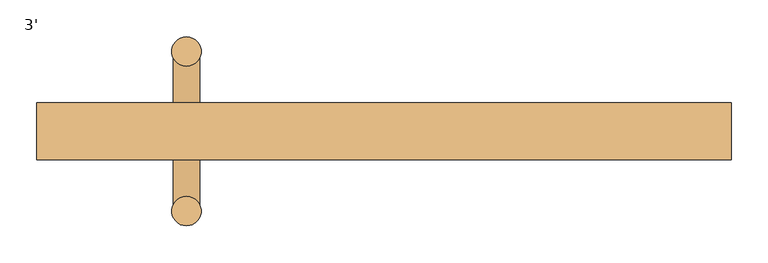
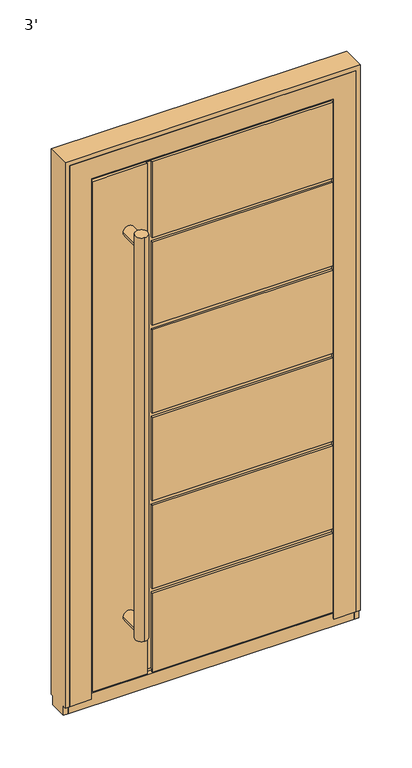
"""IFC4 building model written with IfcOpenShell, lengths in millimetres: door geometry, 3'."""

from ifc_helpers import new_model, si_unit, point, frame, frame_2d, origin, place, context, project, spatial, circle_curve, trimmed, segment, composite_curve, outline, extrude, faceted_brep, source, transform, mapped, element, save


def door_3_ad1505b7(model_context):
    return source(origin(), model_context, "Body", "SolidModel", [
        extrude(outline(composite_curve([segment(trimmed(circle_curve(frame_2d((-268.65, -90.8003001)), 20.0), [point((-268.65, -70.8003001))], [point((-268.65, -110.8003001))], False, "CARTESIAN"), True, "CONTINUOUS"), segment(trimmed(circle_curve(frame_2d((-268.65, -90.8003001)), 20.0), [point((-268.65, -110.8003001))], [point((-268.65, -70.8003001))], False, "CARTESIAN"), True, "CONTINUOUS")], self_intersect=False)), frame((0.0, 0.0, 210.0000003), z_axis=(0.0, 0.0, 1.0), x_axis=(1.0, 0.0, 0.0)), (0.0, 0.0, 1.0), 1363.8),
        extrude(outline(composite_curve([segment(trimmed(circle_curve(frame_2d((-268.65, 126.2003001)), 20.0), [point((-268.65, 146.2003001))], [point((-268.65, 106.2003001))], False, "CARTESIAN"), True, "CONTINUOUS"), segment(trimmed(circle_curve(frame_2d((-268.65, 126.2003001)), 20.0), [point((-268.65, 106.2003001))], [point((-268.65, 146.2003001))], False, "CARTESIAN"), True, "CONTINUOUS")], self_intersect=False)), frame((0.0, 0.0, 210.0000003), z_axis=(0.0, 0.0, 1.0), x_axis=(1.0, 0.0, 0.0)), (0.0, 0.0, 1.0), 1363.8),
        extrude(outline(composite_curve([segment(trimmed(circle_curve(frame_2d((241.9000003, -268.65)), 18.0), [point((241.9000003, -286.65))], [point((241.9000003, -250.65))], False, "CARTESIAN"), True, "CONTINUOUS"), segment(trimmed(circle_curve(frame_2d((241.9000003, -268.65)), 18.0), [point((241.9000003, -250.65))], [point((241.9000003, -286.65))], False, "CARTESIAN"), True, "CONTINUOUS")], self_intersect=False)), frame((0.0, -90.8, 0.0), z_axis=(0.0, 1.0, 0.0), x_axis=(0.0, 0.0, 1.0)), (0.0, 0.0, 1.0), 217.0),
        extrude(outline(composite_curve([segment(trimmed(circle_curve(frame_2d((1541.9000003, -268.65)), 18.0), [point((1541.9000003, -286.65))], [point((1541.9000003, -250.65))], False, "CARTESIAN"), True, "CONTINUOUS"), segment(trimmed(circle_curve(frame_2d((1541.9000003, -268.65)), 18.0), [point((1541.9000003, -250.65))], [point((1541.9000003, -286.65))], False, "CARTESIAN"), True, "CONTINUOUS")], self_intersect=False)), frame((0.0, -90.8, 0.0), z_axis=(0.0, 1.0, 0.0), x_axis=(0.0, 0.0, 1.0)), (0.0, 0.0, 1.0), 217.0),
        faceted_brep([(-193.65, -13.8, 306.466667), (-193.65, -13.8, 587.9333337), (383.65, -13.8, 587.9333337), (383.65, -13.8, 602.9333337), (-193.65, -13.8, 602.9333337), (-193.65, -13.8, 884.4000004), (383.65, -13.8, 884.4000004), (383.65, -13.8, 899.4000004), (-193.65, -13.8, 899.4000004), (-193.65, -13.8, 1180.866667), (383.65, -13.8, 1180.866667), (383.65, -13.8, 1195.866667), (-193.65, -13.8, 1195.866667), (-193.65, -13.8, 1477.3333337), (383.65, -13.8, 1477.3333337), (383.65, -13.8, 1492.3333337), (-193.65, -13.8, 1492.3333337), (-193.65, -13.8, 1748.8000003), (-208.65, -13.8, 1748.8000003), (-208.65, -13.8, 35.0), (-193.65, -13.8, 35.0), (-193.65, -13.8, 291.466667), (383.65, -13.8, 291.466667), (383.65, -13.8, 306.466667), (-193.65, -20.8, 306.466667), (-193.65, -20.8, 587.9333337), (383.65, -20.8, 587.9333337), (383.65, -11.7997698, 1748.8000003), (383.65, -20.8, 1748.8000003), (383.65, -20.8, 1492.3333337), (383.65, -20.8, 1477.3333337), (383.65, -20.8, 1195.866667), (383.65, -20.8, 1180.866667), (383.65, -20.8, 899.4000004), (383.65, -20.8, 884.4000004), (383.65, -20.8, 602.9333337), (383.65, -20.8, 306.466667), (383.65, -20.8, 291.466667), (383.65, -20.8, 24.0), (383.65, -18.8020472, 24.0), (383.65, -18.8020472, 35.0), (383.65, -11.7997698, 35.0), (-193.65, -20.8, 602.9333337), (-193.65, -20.8, 884.4000004), (-193.65, -20.8, 899.4000004), (-193.65, -20.8, 1180.866667), (-208.65, -20.8, 1748.8000003), (-208.65, -20.8, 24.0), (-208.65, -18.8020472, 24.0), (-208.65, -18.8020472, 35.0), (-193.65, -18.8020472, 35.0), (-383.65, -18.8020472, 35.0), (-383.65, -11.7997698, 35.0), (-193.65, -20.8, 291.466667), (-193.65, -18.8020472, 24.0), (-193.65, -20.8, 24.0), (-383.65, -18.8020472, 24.0), (-383.65, -20.8, 24.0), (-383.65, -20.8, 1748.8000003), (-193.65, -20.8, 1477.3333337), (-193.65, -20.8, 1195.866667), (-193.65, -20.8, 1748.8000003), (-193.65, -20.8, 1492.3333337), (408.65, 56.2, 10.0000003), (408.65, 53.2, 10.0000003), (-193.65, 53.2, 10.0000003), (-193.65, 56.2, 10.0000003), (-408.65, 53.2, 10.0000003), (-408.65, 56.2, 10.0000003), (-208.65, 56.2, 10.0000003), (-208.65, 53.2, 10.0000003), (408.65, 56.2, 291.466667), (408.65, 53.2, 291.466667), (408.65, 56.2, 306.466667), (408.65, 56.2, 587.9333337), (408.65, 53.2, 587.9333337), (408.65, 53.2, 306.466667), (408.65, 56.2, 899.4000004), (408.65, 56.2, 1180.866667), (408.65, 53.2, 1180.866667), (408.65, 53.2, 899.4000004), (408.65, 56.2, 602.9333337), (408.65, 56.2, 884.4000004), (408.65, 53.2, 884.4000004), (408.65, 53.2, 602.9333337), (408.65, 56.2, 1195.866667), (408.65, 56.2, 1477.3333337), (408.65, 53.2, 1477.3333337), (408.65, 53.2, 1195.866667), (408.65, 56.2, 1773.8000003), (408.65, 53.2, 1773.8000003), (408.65, 53.2, 1492.3333337), (408.65, 56.2, 1492.3333337), (393.15, 53.2, 291.466667), (393.15, 53.2, 25.5), (-193.65, 53.2, 25.5), (393.15, 53.2, 587.9333337), (393.15, 53.2, 306.466667), (393.15, 53.2, 1180.866667), (393.15, 53.2, 899.4000004), (393.15, 53.2, 884.4000004), (393.15, 53.2, 602.9333337), (393.15, 53.2, 1477.3333337), (393.15, 53.2, 1195.866667), (-193.65, 53.2, 1773.8000003), (-193.65, 53.2, 1758.3000003), (393.15, 53.2, 1758.3000003), (393.15, 53.2, 1492.3333337), (-393.15, 53.2, 25.5), (-393.15, 53.2, 1758.3000003), (-208.65, 53.2, 1758.3000003), (-208.65, 53.2, 1773.8000003), (-408.65, 53.2, 1773.8000003), (-208.65, 53.2, 25.5), (-193.65, 49.2, 291.466667), (-193.65, 56.2, 291.466667), (-193.65, 49.2, 25.5), (-193.65, 56.2, 306.466667), (-193.65, 56.2, 587.9333337), (-193.65, 56.2, 899.4000004), (-193.65, 56.2, 1180.866667), (-193.65, 56.2, 602.9333337), (-193.65, 56.2, 884.4000004), (-193.65, 56.2, 1195.866667), (-193.65, 56.2, 1477.3333337), (-193.65, 56.2, 1492.3333337), (-193.65, 56.2, 1773.8000003), (-408.65, 56.2, 1773.8000003), (-208.65, 56.2, 1773.8000003), (-208.65, 49.2, 1758.3000003), (-208.65, 49.2, 25.5), (-383.65, -11.7997698, 1748.8000003), (393.15, -11.7997698, 1758.3000003), (-393.15, -11.7997698, 1758.3000003), (-393.15, -11.7997698, 25.5), (393.15, -11.7997698, 25.5), (393.15, 49.2, 291.466667), (393.15, 49.2, 306.466667), (393.15, 49.2, 587.9333337), (393.15, 49.2, 602.9333337), (393.15, 49.2, 884.4000004), (393.15, 49.2, 899.4000004), (393.15, 49.2, 1180.866667), (393.15, 49.2, 1195.866667), (393.15, 49.2, 1477.3333337), (393.15, 49.2, 1492.3333337), (-193.65, 49.2, 1477.3333337), (-193.65, 49.2, 1195.866667), (-193.65, 49.2, 1180.866667), (-193.65, 49.2, 899.4000004), (-193.65, 49.2, 884.4000004), (-193.65, 49.2, 602.9333337), (-193.65, 49.2, 587.9333337), (-193.65, 49.2, 306.466667), (-193.65, 49.2, 1758.3000003), (-193.65, 49.2, 1492.3333337)], [[[0, 1, 2, 3, 4, 5, 6, 7, 8, 9, 10, 11, 12, 13, 14, 15, 16, 17, 18, 19, 20, 21, 22, 23]], [[1, 0, 24, 25]], [[1, 25, 26, 2]], [[27, 28, 29, 15, 14, 30, 31, 11, 10, 32, 33, 7, 6, 34, 35, 3, 2, 26, 36, 23, 22, 37, 38, 39, 40, 41]], [[42, 4, 3, 35]], [[5, 4, 42, 43]], [[5, 43, 34, 6]], [[44, 8, 7, 33]], [[9, 8, 44, 45]], [[19, 18, 46, 47, 48, 49]], [[41, 40, 50, 20, 19, 49, 51, 52]], [[53, 21, 20, 50, 54, 55]], [[21, 53, 37, 22]], [[24, 0, 23, 36]], [[40, 39, 54, 50]], [[56, 51, 49, 48]], [[39, 38, 55, 54]], [[57, 56, 48, 47]], [[33, 32, 45, 44]], [[35, 34, 43, 42]], [[36, 26, 25, 24]], [[55, 38, 37, 53]], [[58, 57, 47, 46]], [[31, 30, 59, 60]], [[28, 61, 62, 29]], [[63, 64, 65, 66]], [[67, 68, 69, 70]], [[64, 63, 71, 72]], [[73, 74, 75, 76]], [[77, 78, 79, 80]], [[81, 82, 83, 84]], [[85, 86, 87, 88]], [[89, 90, 91, 92]], [[65, 64, 72, 93, 94, 95]], [[76, 75, 96, 97]], [[80, 79, 98, 99]], [[84, 83, 100, 101]], [[88, 87, 102, 103]], [[90, 104, 105, 106, 107, 91]], [[108, 109, 110, 111, 112, 67, 70, 113]], [[114, 115, 66, 65, 95, 116]], [[63, 66, 115, 71]], [[74, 73, 117, 118]], [[78, 77, 119, 120]], [[82, 81, 121, 122]], [[86, 85, 123, 124]], [[89, 92, 125, 126]], [[68, 127, 128, 69]], [[68, 67, 112, 127]], [[129, 130, 113, 70, 69, 128, 111, 110]], [[58, 131, 52, 51, 56, 57]], [[132, 133, 134, 135], [131, 27, 41, 52]], [[106, 132, 135, 94, 93, 136, 137, 97, 96, 138, 139, 101, 100, 140, 141, 99, 98, 142, 143, 103, 102, 144, 145, 107]], [[94, 135, 134, 108, 113, 130, 116, 95]], [[133, 109, 108, 134]], [[146, 147, 143, 142, 148, 149, 141, 140, 150, 151, 139, 138, 152, 153, 137, 136, 114, 116, 130, 129, 154, 155, 145, 144]], [[149, 148, 120, 119]], [[149, 119, 77, 80, 99, 141]], [[122, 150, 140, 100, 83, 82]], [[151, 150, 122, 121]], [[151, 121, 81, 84, 101, 139]], [[118, 152, 138, 96, 75, 74]], [[153, 152, 118, 117]], [[153, 117, 73, 76, 97, 137]], [[115, 114, 136, 93, 72, 71]], [[9, 45, 32, 10]], [[60, 12, 11, 31]], [[13, 12, 60, 59]], [[13, 59, 30, 14]], [[62, 16, 15, 29]], [[16, 62, 61, 17]], [[124, 146, 144, 102, 87, 86]], [[125, 155, 154, 105, 104, 126]], [[120, 148, 142, 98, 79, 78]], [[147, 123, 85, 88, 103, 143]], [[147, 146, 124, 123]], [[155, 125, 92, 91, 107, 145]], [[90, 89, 126, 104]], [[127, 112, 111, 128]], [[132, 106, 105, 154, 129, 110, 109, 133]], [[27, 131, 58, 46, 18, 17, 61, 28]]]),
        faceted_brep([(-457.2, 56.2, 0.0), (-412.7, 56.2, 0.0), (-412.7, 47.2, 0.0), (-457.2, 47.1997571, 0.0), (-403.2, -16.2999958, 0.0), (-387.7, -16.2999958, 0.0), (-387.7, -20.8, 0.0), (-457.2, -20.8, 0.0), (-457.2, -11.8, 0.0), (-403.2, -11.8, 0.0), (457.2, -20.8, 0.0), (387.7, -20.8, 0.0), (387.7, -16.2999958, 0.0), (403.2, -16.2999958, 0.0), (403.2, -11.8, 0.0), (457.2, -11.8, 0.0), (412.7, 47.2, 0.0), (412.7, 56.2, 0.0), (457.2, 56.2, 0.0), (457.2, 47.1997571, 0.0), (-457.2, -20.8, 1828.8), (-457.2, 56.2, 1828.8), (-457.2, 47.1997571, -30.0), (-457.2, -11.8, -30.0), (457.2, 56.2, 1828.8), (412.7, 56.2, 1784.3), (-412.7, 56.2, 1784.3), (457.2, -20.8, 1828.8), (457.2, -11.8, -30.0), (457.2, 47.1997571, -30.0), (-387.7, -20.8, 1759.3), (387.7, -20.8, 1759.3), (-403.2, 47.2, 1774.8), (-403.2, -16.2999958, 1774.8), (-403.2, -11.8, 14.5), (-403.2, 47.2, 14.5), (403.2, 47.2, 1774.8), (403.2, -16.2999958, 1774.8), (403.2, 47.2, 14.5), (403.2, -11.8, 14.5), (-412.7, 47.2, 1784.3), (412.7, 47.2, 1784.3), (387.7, -16.2999958, 1759.3), (-387.7, -16.2999958, 1759.3)], [[[0, 1, 2, 3]], [[4, 5, 6, 7, 8, 9]], [[10, 11, 12, 13, 14, 15]], [[16, 17, 18, 19]], [[7, 20, 21, 0, 3, 22, 23, 8]], [[1, 0, 21, 24, 18, 17, 25, 26]], [[21, 20, 27, 24]], [[18, 24, 27, 10, 15, 28, 29, 19]], [[7, 6, 30, 31, 11, 10, 27, 20]], [[32, 33, 4, 9, 34, 35]], [[33, 32, 36, 37]], [[37, 36, 38, 39, 14, 13]], [[40, 2, 1, 26]], [[16, 19, 29, 22, 3, 2, 40, 41], [36, 32, 35, 38]], [[5, 4, 33, 37, 13, 12, 42, 43]], [[6, 5, 43, 30]], [[26, 25, 41, 40]], [[31, 30, 43, 42]], [[17, 16, 41, 25]], [[12, 11, 31, 42]], [[23, 28, 15, 14, 39, 34, 9, 8]], [[38, 35, 34, 39]], [[23, 22, 29, 28]]]),
        faceted_brep([(-457.2, 47.2, -30.0), (-457.2, -11.8, -30.0), (-472.2, -11.8, -30.0), (-472.2, 47.2, -30.0), (-457.2, 56.2, 1828.8), (-457.2, -20.8, 1828.8), (-457.2, -20.8, 0.0), (-457.2, -11.8, 0.0), (-457.2, 47.2, 0.0), (-457.2, 56.2, 0.0), (472.2, -11.8, 0.0), (457.2, -11.8, 0.0), (457.2, -11.8, -30.0), (472.2, -11.8, -30.0), (-472.2, -11.8, 0.0), (-472.2, -20.8, 1843.8), (-472.2, 56.2, 1843.8), (-472.2, 56.2, 0.0), (-472.2, 47.2, 0.0), (-472.2, -20.8, 0.0), (457.2, 47.2, 0.0), (472.2, 47.2, 0.0), (472.2, 47.2, -30.0), (457.2, 47.2, -30.0), (457.2, -20.8, 1828.8), (457.2, 56.2, 1828.8), (457.2, 56.2, 0.0), (457.2, -20.8, 0.0), (472.2, 56.2, 1843.8), (472.2, 56.2, 0.0), (472.2, -20.8, 0.0), (472.2, -20.8, 1843.8)], [[[0, 1, 2, 3]], [[4, 5, 6, 7, 1, 0, 8, 9]], [[10, 11, 12, 13]], [[7, 14, 2, 1]], [[15, 16, 17, 18, 3, 2, 14, 19]], [[20, 21, 22, 23]], [[18, 8, 0, 3]], [[24, 25, 26, 20, 23, 12, 11, 27]], [[25, 4, 9, 17, 16, 28, 29, 26]], [[21, 20, 26, 29]], [[8, 18, 17, 9]], [[22, 13, 12, 23]], [[11, 10, 30, 27]], [[14, 7, 6, 19]], [[5, 24, 27, 30, 31, 15, 19, 6]], [[28, 31, 30, 10, 13, 22, 21, 29]], [[5, 4, 25, 24]], [[16, 15, 31, 28]]]),
    ])


if __name__ == "__main__":
    model = new_model("IFC4")
    model_context = context("Model", 3, world=origin())
    ifc_project = project(units=[si_unit("LENGTHUNIT", "METRE", prefix="MILLI")], contexts=[model_context])
    site = spatial("IfcSite", under=ifc_project)
    building = spatial("IfcBuilding", under=site)
    placement = place(None, origin())
    door_3_shape = door_3_ad1505b7(model_context)
    element("IfcDoor", 1, ObjectType="3'", at=placement, inside=building, context=model_context, shape_type="MappedRepresentation", body=[
        mapped(door_3_shape, transform((0.0, 0.0, 0.0), x_axis=(1.0, 0.0, 0.0), y_axis=(0.0, 1.0, 0.0), z_axis=(0.0, 0.0, 1.0))),
    ])
    save(model, "model.ifc")

# Revit data of these elements
# Type "3'"
#   Type Mark = "41"
#   Water resistance = "up to Class E900, EN 12208:2001"
#   Uniclass2015Version = "v1.21"
#   Uniclass2015Reference = "Ss_25_30_20_30"
#   Uniclass2015Description = "Frame and door leaf system"
#   URL = "www.aluprof.com"
#   Type IFC Predefined Type = "USERDEFINED"
#   Right-hand / Left-hand door [instance default] = ""
#   Resistance to wind load = "up to Class C5/B5, EN 12210:2001"
#   Insert type = "ST"
#   Hardware [instance default] = ""
#   Product page = "https://aluprof.com/en/architects/offer/window-and-door-systems/panel-doors#visualisation"
#   Operation = "SinglePanelOutwardOpening"
#   Opening type = "Outward"
#   NBSReference = "25-50-20/125"
#   NBSDescription = "Frame and door leaf system"
#   Important = "The actual acceptable construction dimensions are dependent on the selection of profiles and hardware, glazing type, construction weight and the construction’s operating conditions. These should be determined by a suitably qualified person, and using ALUPROF’s calculation software"
#   IfcExportType = "USERDEFINED"
#   IfcExportAs = "IfcDoorType"
#   Handle type [instance default] = ""
#   Manufacturer = "ALUPROF SA"
#   Export Type to IFC As = "IfcDoorType"
#   Door sill type [instance default] = ""
#   Description = "External single-leaf panel door outward opening"
#   Model = "MB-86 ST Panel Door AD07"
#   Content of the recyclate in the material = "69.2%"
#   COBie.Type.WarrantyDurationParts = ""
#   COBie.Type.Name = ""
#   COBie.Type.Manufacturer = "ALUPROF SA"
#   COBie.Space.Name = ""
#   COBie.Floor.Name = ""
#   COBie.Facility.Name = ""
#   COBie.CreatedOn = ""
#   COBie.Component.WarrantyStartDate = ""
#   COBie.Component.Name = "MB-86 ST Panel Door AD07"
#   Burglar resistance = "RC2"
#   Air permeability = "up to Class 4, EN 12207:2001"
#   Width of the active leaf = 2' - 8.17717"
#   Placement in wall = 0' - 0.7874"
#   Thickness = 0' - 3.0315"
#   Height of the opening sash = 5' - 9.44094"
#   Handle Offset = 3' - 5.33858"
#   Rough Height = 6' - 2.40945"
#   Rough Width = 3' - 1.1811"
#   Height = 6' - 0"
#   Width = 3' - 0"
#   Construction depth = 0' - 3.0315"
#   Clear opening width = 2' - 3.94882"
#   Clear opening height = 5' - 8.47638"
#   Height of the array = 0' - 11.08136"
#   Schedule No. [instance default] = 1
#   Handrail [instance default] = yes
#   IsExternal = yes
#   Handle [instance default] = no
#   Door closer [instance default] = no
#   Function = 1
#   COBie.Type = yes
#   COBie = yes
#   Access control [instance default] = no
#   Panel = element 371215
#   Wall Closure = (empty or 0)
